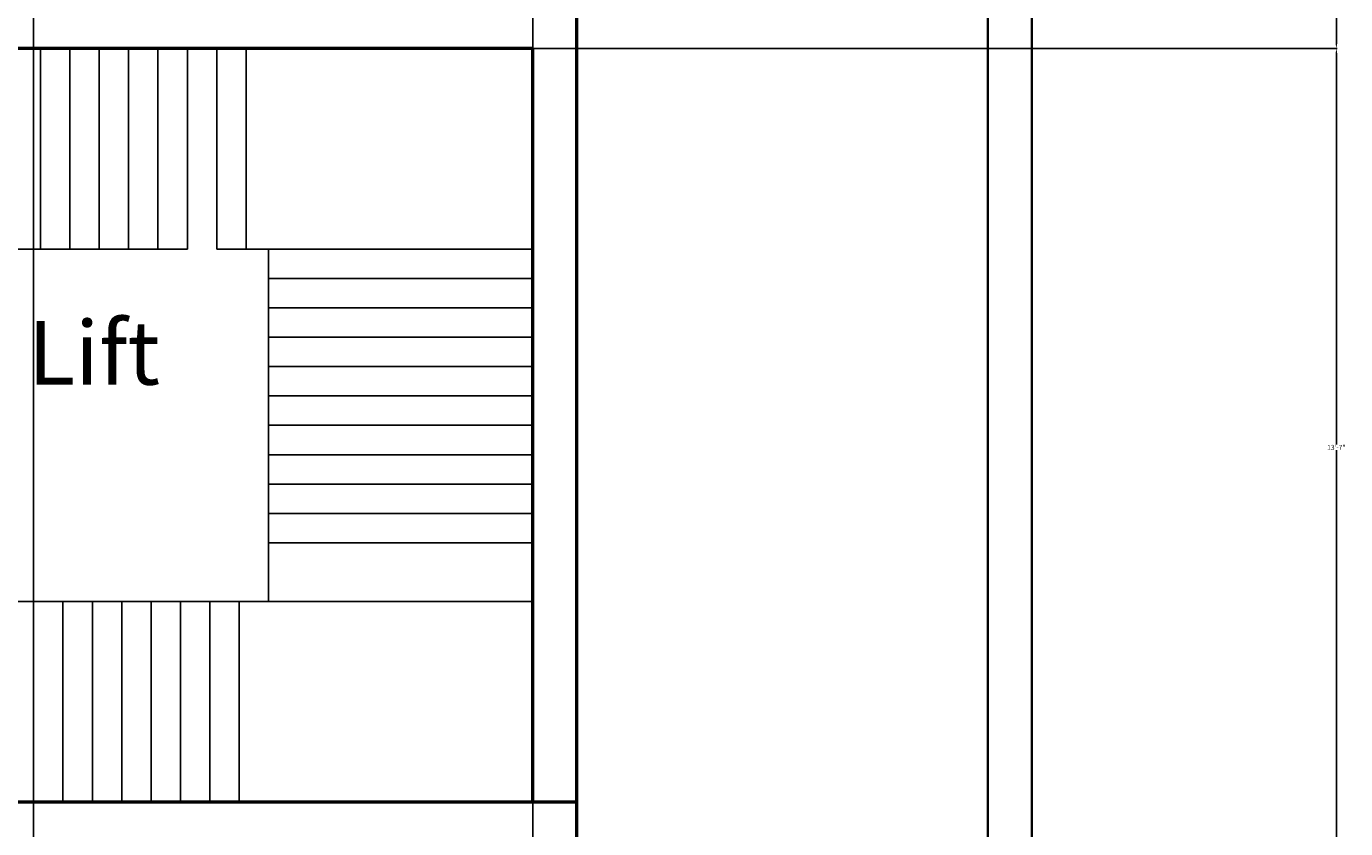
# Model space of a CAD drawing. Units: inches. Extents: x -364 to 705, y -52 to 1250.
# Tile 14 of 34: x 435 to 705, y 144 to 308. Entities that reach past the tile are written whole.
import ezdxf

# ---------------------------------------------------------------- set-up
doc = ezdxf.new("R2010")
doc.units = ezdxf.units.IN
doc.header["$MEASUREMENT"] = 0
for name, color, linetype, lineweight in [('A-ANNO-DIMS', 4, 'Continuous', 18), ('A-AREA-IDEN', 3, 'Continuous', 18), ('A-FLOR-STRS', 7, 'Continuous', 25), ('A-WALL', 41, 'Continuous', 50), ('C-WALL', 41, 'Continuous', 35)]:
    doc.layers.add(name, color=color, linetype=linetype, lineweight=lineweight)
doc.styles.get("Standard").update_dxf_attribs({"font": 'arial.ttf'})
doc.dimstyles.get("Standard").update_dxf_attribs({"dimtxt": 1, "dimasz": 1, "dimexe": 0.18, "dimexo": 0.0625, "dimgap": 0.09, "dimtad": 0, "dimtih": 1, "dimtoh": 1, "dimdec": 0, "dimzin": 0, "dimdsep": 46, "dimlunit": 3, "dimtxsty": 'Standard', "dimcen": 0.09, "dimadec": 0, "dimazin": 0, "dimtfac": 1, "dimtdec": 0, "dimtofl": 0, "dimtmove": 0, "dimatfit": 3, "dimfxl": 1, "dimtolj": 1, "dimtzin": 0, "dimarcsym": 0})

# ---------------------------------------------------------------- blocks, each defined once
blk = doc.blocks.new('*D78')
at = {"layer": 'A-ANNO-DIMS', "color": 0, "lineweight": -2, "transparency": 16777216}
for p, q in [((538.64, 303.11), (703.01, 303.11)), ((702.83, 302.11), (702.83, 222.22)), ((702.83, 141.11), (702.83, 221.01)), ((538.64, 140.11), (703.01, 140.11))]:
    blk.add_line(p, q, dxfattribs=at)
at = {"layer": 'A-ANNO-DIMS', "color": 0, "transparency": 16777216}
for points in [[(702.66, 302.11), (703, 302.11), (702.83, 303.11)], [(702.66, 141.11), (703, 141.11), (702.83, 140.11)]]:
    blk.add_solid(points, dxfattribs=at)
at = {"layer": 'Defpoints', "color": 0, "transparency": 16777216}
for p in [(538.58, 303.11), (702.83, 303.11), (538.58, 140.11)]:
    blk.add_point(p, dxfattribs=at)
at = {"layer": 'A-ANNO-DIMS', "color": 0, "transparency": 16777216, "insert": (702.83, 221.61), "char_height": 1, "attachment_point": 5}
blk.add_mtext('\\A1;13\'-7"', dxfattribs=at)
blk = doc.blocks.new('*D79')
at = {"layer": 'A-ANNO-DIMS', "color": 0, "lineweight": -2, "transparency": 16777216}
for p, q in [((538.64, 408.11), (703.01, 408.11)), ((702.83, 407.11), (702.83, 356.22)), ((702.83, 304.11), (702.83, 355.01)), ((538.64, 303.11), (703.01, 303.11))]:
    blk.add_line(p, q, dxfattribs=at)
at = {"layer": 'A-ANNO-DIMS', "color": 0, "transparency": 16777216}
for points in [[(702.66, 407.11), (703, 407.11), (702.83, 408.11)], [(702.66, 304.11), (703, 304.11), (702.83, 303.11)]]:
    blk.add_solid(points, dxfattribs=at)
at = {"layer": 'Defpoints', "color": 0, "transparency": 16777216}
for p in [(538.58, 408.11), (702.83, 408.11), (538.58, 303.11)]:
    blk.add_point(p, dxfattribs=at)
at = {"layer": 'A-ANNO-DIMS', "color": 0, "transparency": 16777216, "insert": (702.83, 355.61), "char_height": 1, "attachment_point": 5}
blk.add_mtext('\\A1;8\'-9"', dxfattribs=at)
blk = doc.blocks.new('*D100')
at = {"layer": 'A-ANNO-DIMS', "color": 0, "lineweight": -2, "transparency": 16777216}
for p, q in [((436.58, 417.05), (436.58, -51.32)), ((538.58, 417.05), (538.58, -51.32)), ((437.58, -51.14), (486.16, -51.14)), ((537.58, -51.14), (489, -51.14))]:
    blk.add_line(p, q, dxfattribs=at)
at = {"layer": 'A-ANNO-DIMS', "color": 0, "transparency": 16777216}
for points in [[(437.58, -50.97), (437.58, -51.3), (436.58, -51.14)], [(537.58, -50.97), (537.58, -51.3), (538.58, -51.14)]]:
    blk.add_solid(points, dxfattribs=at)
at = {"layer": 'Defpoints', "color": 0, "transparency": 16777216}
for p in [(436.58, 417.11), (538.58, 417.11), (538.58, -51.14)]:
    blk.add_point(p, dxfattribs=at)
at = {"layer": 'A-ANNO-DIMS', "color": 0, "transparency": 16777216, "insert": (487.58, -51.14), "char_height": 1, "attachment_point": 5}
blk.add_mtext('\\A1;8\'-6"', dxfattribs=at)

msp = doc.modelspace()

# ---------------------------------------------------------------- linework, layer by layer
at = {"layer": 'A-FLOR-STRS'}
for p, q in [((438, 303.11), (438, 262.11)), ((444, 303.11), (444, 262.11)), ((450, 303.11), (450, 262.11)), ((456, 303.11), (456, 262.11)), ((462, 303.11), (462, 262.11)), ((468, 303.11), (468, 262.11)), ((474, 303.11), (474, 262.11)), ((480, 303.11), (480, 262.11)), ((412.58, 262.11), (468, 262.11)), ((474, 262.11), (538.58, 262.11)), ((484.58, 190.11), (484.58, 262.11)), ((484.58, 256.11), (538.58, 256.11)), ((484.58, 250.11), (538.58, 250.11)), ((484.58, 244.11), (538.58, 244.11)), ((484.58, 238.11), (538.58, 238.11)), ((484.58, 232.11), (538.58, 232.11)), ((484.58, 226.11), (538.58, 226.11)), ((484.58, 220.11), (538.58, 220.11)), ((484.58, 214.11), (538.58, 214.11)), ((484.58, 208.11), (538.58, 208.11)), ((484.58, 208.11), (538.58, 208.11)), ((484.58, 202.11), (538.58, 202.11)), ((412.58, 190.11), (538.58, 190.11)), ((436.58, 190.11), (436.58, 149.11)), ((442.58, 190.11), (442.58, 149.11)), ((448.58, 190.11), (448.58, 149.11)), ((454.58, 190.11), (454.58, 149.11)), ((460.58, 190.11), (460.58, 149.11)), ((466.58, 190.11), (466.58, 149.11)), ((472.58, 190.11), (472.58, 149.11)), ((478.58, 190.11), (478.58, 149.11))]:
    msp.add_line(p, q, dxfattribs=at)
at = {"layer": 'A-WALL'}
for p, q in [((547.58, 11.11), (547.58, 986.11)), ((538.58, 303.11), (358.58, 303.11)), ((538.58, 149.11), (538.58, 303.11)), ((547.58, 149.11), (412.58, 149.11))]:
    msp.add_line(p, q, dxfattribs=at)
at = {"layer": 'C-WALL'}
for p, q in [((640.58, 11.11), (640.58, 1079.11)), ((631.58, 11.11), (631.58, 1070.11))]:
    msp.add_line(p, q, dxfattribs=at)

# ---------------------------------------------------------------- texts
at = {"layer": 'A-AREA-IDEN', "insert": (435.44, 247.42), "char_height": 13, "attachment_point": 1}
msp.add_mtext_dynamic_manual_height_columns('Lift', width=30.2774, gutter_width=1, heights=[0], dxfattribs=at)

# ---------------------------------------------------------------- dimensions: what is measured, and where the dimension line sits
at = {"layer": 'A-ANNO-DIMS'}
dim = msp.add_linear_dim(base=(538.58, -51.14), p1=(436.58, 417.11), p2=(538.58, 417.11), dimstyle='Standard', override={"dimdec": 1, "dimlfac": 1, "dimrnd": 0, "dimzin": 1, "dimdsep": 46, "dimlunit": 4, "dimfrac": 2}, dxfattribs=at)
dim.commit()
dim.dimension.update_dxf_attribs({"geometry": '*D100', "text_midpoint": (487.58, -51.14)})
for base, p1, p2, picture, middle in [((702.83, 408.11), (538.58, 303.11), (538.58, 408.11), '*D79', (702.83, 355.61)), ((702.83, 303.11), (538.58, 140.11), (538.58, 303.11), '*D78', (702.83, 221.61))]:
    dim = msp.add_linear_dim(base=base, p1=p1, p2=p2, angle=90, dimstyle='Standard', override={"dimdec": 1, "dimlfac": 1, "dimrnd": 0, "dimzin": 1, "dimdsep": 46, "dimlunit": 4, "dimfrac": 2}, dxfattribs=at)
    dim.commit()
    dim.dimension.update_dxf_attribs({"geometry": picture, "text_midpoint": middle})

doc.saveas('drawing.dxf')
